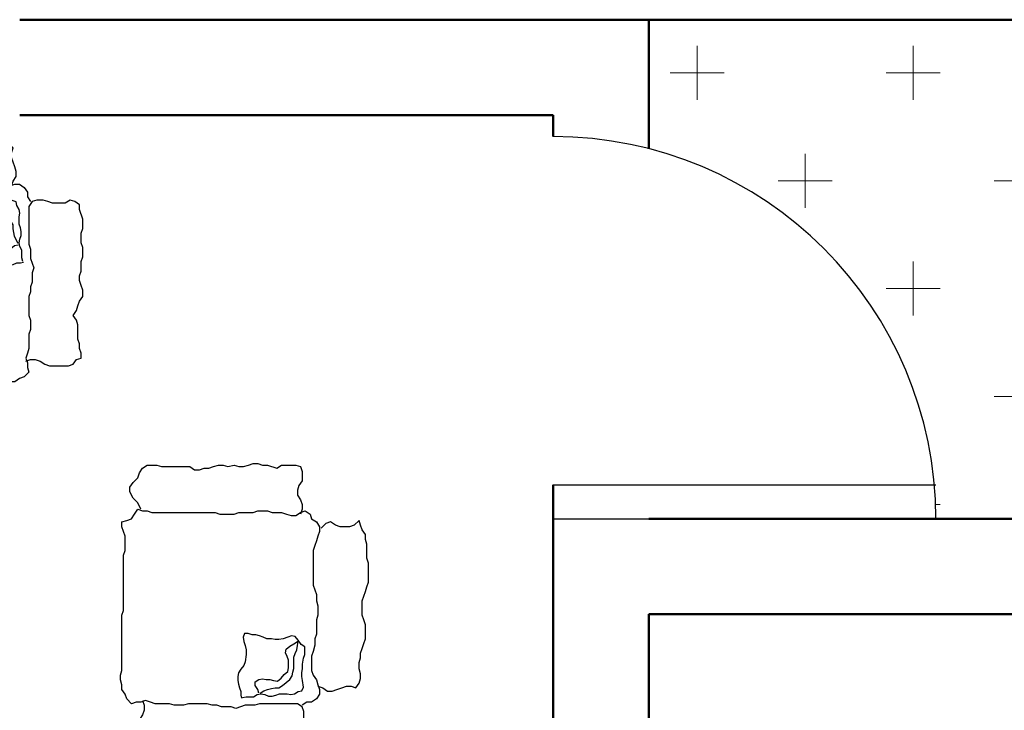
# Model space of a CAD drawing. Units: millimetres. Extents: x -857 to 54106, y -13666 to 13947.
# Tile 28 of 41: x 28540 to 30856, y 11178 to 12804. Entities that reach past the tile are written whole.
import ezdxf

# ---------------------------------------------------------------- set-up
doc = ezdxf.new("R2010")
doc.units = ezdxf.units.MM
for name, color, linetype, lineweight in [('A-DOOR', 1, 'Continuous', 25), ('A-FLOR-PATT', 252, 'Continuous', 13), ('A-FURN', 21, 'Continuous', 18), ('A-WALL', 7, 'Continuous', 50)]:
    doc.layers.add(name, color=color, linetype=linetype, lineweight=lineweight)
doc.layers.add('TEFRIŞ', color=11, linetype='Continuous')

# ---------------------------------------------------------------- blocks, each defined once
blk = doc.blocks.new('24')
at = {"layer": 'TEFRIŞ'}
for p, q in [((-1851.9, -153.78), (-1851.9, -152.78)), ((-1851.9, -152.78), (-1850.24, -152.78)), ((-1849.09, -151.25), (-1850.56, -152.23)), ((-1850.24, -152.78), (-1850.24, -152.11)), ((-1847.61, -151.25), (-1849.09, -151.25)), ((-1846.13, -150.75), (-1847.61, -151.25)), ((-1841.7, -150.75), (-1846.13, -150.75)), ((-1840.23, -150.26), (-1841.7, -150.75)), ((-1834.32, -150.26), (-1840.23, -150.26)), ((-1832.84, -150.75), (-1834.32, -150.26)), ((-1831.36, -151.25), (-1832.84, -150.75)), ((-1829.89, -151.74), (-1831.36, -151.25)), ((-1828.41, -152.23), (-1829.89, -151.74)), ((-1823.98, -152.23), (-1828.41, -152.23)), ((-1822.5, -151.74), (-1823.98, -152.23)), ((-1821.03, -151.25), (-1822.5, -151.74)), ((-1816.6, -151.25), (-1821.03, -151.25)), ((-1815.12, -151.74), (-1816.6, -151.25)), ((-1813.64, -152.23), (-1815.12, -151.74)), ((-1812.17, -152.72), (-1813.64, -152.23)), ((-1810.69, -152.72), (-1812.17, -152.72)), ((-1809.21, -153.21), (-1810.69, -152.72)), ((-1807.24, -153.21), (-1809.21, -153.21)), ((-1805.77, -152.72), (-1807.24, -153.21)), ((-1804.29, -152.72), (-1805.77, -152.72)), ((-1802.81, -153.21), (-1804.29, -152.72)), ((-1802.01, -153.28), (-1802.01, -152.88)), ((-1802.01, -152.88), (-1801, -152.88)), ((-1801, -152.88), (-1801, -152.68)), ((-1801, -152.68), (-1800, -152.68)), ((-1800, -152.68), (-1800, -152.48)), ((-1800, -152.48), (-1797.79, -152.48)), ((-1797.79, -152.48), (-1797.79, -152.68)), ((-1797.79, -152.68), (-1796.79, -152.68)), ((-1796.79, -152.68), (-1796.79, -153.08)), ((-1796.79, -153.08), (-1795.78, -153.08)), ((-1795.78, -153.08), (-1795.78, -152.68)), ((-1795.78, -152.68), (-1794.78, -152.68)), ((-1794.78, -152.68), (-1794.78, -152.08)), ((-1794.78, -152.08), (-1792.77, -152.08)), ((-1792.77, -152.08), (-1792.77, -152.68)), ((-1792.77, -152.68), (-1792.57, -152.68)), ((-1792.5, -152.78), (-1790.84, -152.78)), ((-1792.5, -153.78), (-1792.5, -152.78)), ((-1789.69, -151.25), (-1791.16, -152.23)), ((-1790.84, -152.78), (-1790.84, -152.11)), ((-1788.21, -151.25), (-1789.69, -151.25)), ((-1786.73, -150.75), (-1788.21, -151.25)), ((-1782.3, -150.75), (-1786.73, -150.75)), ((-1780.83, -150.26), (-1782.3, -150.75)), ((-1774.92, -150.26), (-1780.83, -150.26)), ((-1773.44, -150.75), (-1774.92, -150.26)), ((-1771.96, -151.25), (-1773.44, -150.75)), ((-1770.49, -151.74), (-1771.96, -151.25)), ((-1769.01, -152.23), (-1770.49, -151.74)), ((-1764.58, -152.23), (-1769.01, -152.23)), ((-1763.1, -151.74), (-1764.58, -152.23)), ((-1761.63, -151.25), (-1763.1, -151.74)), ((-1757.2, -151.25), (-1761.63, -151.25)), ((-1755.72, -151.74), (-1757.2, -151.25)), ((-1754.24, -152.23), (-1755.72, -151.74)), ((-1752.77, -152.72), (-1754.24, -152.23)), ((-1751.29, -152.72), (-1752.77, -152.72)), ((-1749.81, -153.21), (-1751.29, -152.72)), ((-1747.84, -153.21), (-1749.81, -153.21)), ((-1746.37, -152.72), (-1747.84, -153.21)), ((-1744.89, -152.72), (-1746.37, -152.72)), ((-1743.41, -153.21), (-1744.89, -152.72)), ((-1741.94, -154.2), (-1743.41, -153.21)), ((-1733.14, -152.78), (-1733.14, -153.45)), ((-1732.14, -152.78), (-1733.14, -152.78)), ((-1732.14, -152.45), (-1732.14, -152.78)), ((-1730.14, -152.45), (-1732.14, -152.45)), ((-1728.32, -151.25), (-1729.8, -152.23)), ((-1726.85, -151.25), (-1728.32, -151.25)), ((-1725.37, -150.75), (-1726.85, -151.25)), ((-1720.94, -150.75), (-1725.37, -150.75)), ((-1719.46, -150.26), (-1720.94, -150.75)), ((-1713.56, -150.26), (-1719.46, -150.26)), ((-1712.08, -150.75), (-1713.56, -150.26)), ((-1710.6, -151.25), (-1712.08, -150.75)), ((-1709.12, -151.74), (-1710.6, -151.25)), ((-1707.65, -152.23), (-1709.12, -151.74)), ((-1703.22, -152.23), (-1707.65, -152.23)), ((-1701.74, -151.74), (-1703.22, -152.23)), ((-1700.26, -151.25), (-1701.74, -151.74)), ((-1695.83, -151.25), (-1700.26, -151.25)), ((-1694.36, -151.74), (-1695.83, -151.25)), ((-1692.88, -152.23), (-1694.36, -151.74)), ((-1691.4, -152.72), (-1692.88, -152.23)), ((-1689.93, -152.72), (-1691.4, -152.72)), ((-1688.45, -153.21), (-1689.93, -152.72)), ((-1686.48, -153.21), (-1688.45, -153.21)), ((-1685, -152.72), (-1686.48, -153.21)), ((-1683.53, -152.72), (-1685, -152.72)), ((-1682.05, -153.21), (-1683.53, -152.72)), ((-1680.57, -154.2), (-1682.05, -153.21)), ((-1852.57, -156.78), (-1852.57, -155.78)), ((-1852.57, -155.78), (-1852.24, -155.78)), ((-1852.24, -155.78), (-1852.24, -153.78)), ((-1852.24, -153.78), (-1851.9, -153.78)), ((-1803.01, -153.28), (-1802.01, -153.28)), ((-1793.17, -155.78), (-1792.84, -155.78)), ((-1793.17, -156.78), (-1793.17, -155.78)), ((-1792.84, -155.78), (-1792.84, -153.78)), ((-1792.84, -153.78), (-1792.5, -153.78)), ((-1741.14, -154.45), (-1741.14, -154.11)), ((-1740.14, -154.45), (-1741.14, -154.45)), ((-1740.14, -155.11), (-1740.14, -154.45)), ((-1739.14, -155.11), (-1740.14, -155.11)), ((-1739.14, -155.45), (-1739.14, -155.11)), ((-1738.14, -155.45), (-1739.14, -155.45)), ((-1738.14, -155.11), (-1738.14, -155.45)), ((-1737.14, -155.11), (-1738.14, -155.11)), ((-1737.14, -154.45), (-1737.14, -155.11)), ((-1736.14, -154.45), (-1737.14, -154.45)), ((-1737.14, -155.45), (-1737.14, -155.11)), ((-1736.81, -155.45), (-1737.14, -155.45)), ((-1736.81, -157.45), (-1736.81, -155.45)), ((-1735.14, -154.11), (-1736.14, -154.11)), ((-1736.14, -154.11), (-1736.14, -154.45)), ((-1735.14, -153.78), (-1735.14, -154.11)), ((-1734.14, -153.78), (-1735.14, -153.78)), ((-1734.14, -153.45), (-1734.14, -153.78)), ((-1733.14, -153.45), (-1734.14, -153.45)), ((-1681.06, -155.67), (-1680.57, -154.2)), ((-1681.06, -157.15), (-1681.06, -155.67)), ((-1852.24, -156.78), (-1852.57, -156.78)), ((-1852.24, -158.78), (-1852.24, -156.78)), ((-1851.9, -158.78), (-1852.24, -158.78)), ((-1851.9, -162.78), (-1851.9, -158.78)), ((-1792.84, -156.78), (-1793.17, -156.78)), ((-1792.84, -158.78), (-1792.84, -156.78)), ((-1792.5, -158.78), (-1792.84, -158.78)), ((-1792.5, -162.78), (-1792.5, -158.78)), ((-1736.14, -157.45), (-1736.81, -157.45)), ((-1736.14, -158.45), (-1736.14, -157.45)), ((-1735.81, -158.45), (-1736.14, -158.45)), ((-1735.81, -160.11), (-1735.81, -158.45)), ((-1680.57, -158.63), (-1681.06, -157.15)), ((-1680.08, -160.1), (-1680.57, -158.63)), ((-1734.48, -160.11), (-1735.81, -160.11)), ((-1735.14, -162.11), (-1734.48, -162.11)), ((-1735.14, -163.11), (-1735.14, -162.11)), ((-1734.48, -162.11), (-1734.48, -160.11)), ((-1679.59, -161.58), (-1680.08, -160.1)), ((-1679.59, -163.05), (-1679.59, -161.58)), ((-1851.57, -162.78), (-1851.9, -162.78)), ((-1851.9, -166.44), (-1851.9, -165.44)), ((-1851.9, -165.44), (-1850.9, -165.44)), ((-1851.57, -164.78), (-1851.57, -162.78)), ((-1850.57, -164.78), (-1851.57, -164.78)), ((-1850.9, -165.44), (-1850.9, -164.78)), ((-1850.57, -165.44), (-1850.57, -164.78)), ((-1849.57, -165.44), (-1850.57, -165.44)), ((-1792.17, -162.78), (-1792.5, -162.78)), ((-1792.5, -165.44), (-1791.5, -165.44)), ((-1792.5, -166.44), (-1792.5, -165.44)), ((-1792.17, -164.78), (-1792.17, -162.78)), ((-1791.17, -164.78), (-1792.17, -164.78)), ((-1791.5, -165.44), (-1791.5, -164.78)), ((-1791.17, -165.44), (-1791.17, -164.78)), ((-1790.17, -165.44), (-1791.17, -165.44)), ((-1742.48, -164.78), (-1740.81, -164.78)), ((-1742.48, -165.78), (-1742.48, -164.78)), ((-1740.81, -164.11), (-1738.81, -164.11)), ((-1740.81, -164.78), (-1740.81, -164.11)), ((-1738.81, -164.11), (-1738.81, -164.45)), ((-1738.81, -164.45), (-1737.81, -164.45)), ((-1737.81, -164.45), (-1737.81, -164.78)), ((-1737.81, -164.78), (-1736.81, -164.78)), ((-1736.81, -164.78), (-1736.81, -165.11)), ((-1736.81, -165.11), (-1735.81, -165.11)), ((-1735.81, -165.44), (-1736.14, -165.44)), ((-1735.81, -163.11), (-1735.14, -163.11)), ((-1735.81, -165.11), (-1735.81, -163.11)), ((-1735.81, -165.11), (-1735.81, -165.44)), ((-1734.14, -165.11), (-1733.14, -165.11)), ((-1734.14, -165.78), (-1734.14, -165.11)), ((-1733.14, -164.78), (-1731.14, -164.78)), ((-1733.14, -165.11), (-1733.14, -164.78)), ((-1731.14, -164.78), (-1731.14, -165.11)), ((-1731.14, -165.11), (-1730.14, -165.11)), ((-1730.14, -165.11), (-1730.14, -165.44)), ((-1730.14, -165.44), (-1727.81, -165.44)), ((-1681.06, -166), (-1680.57, -164.53)), ((-1680.57, -164.53), (-1679.59, -163.05)), ((-1853.9, -169.44), (-1853.9, -168.44)), ((-1853.9, -168.44), (-1852.57, -168.44)), ((-1852.57, -168.44), (-1852.57, -166.44)), ((-1852.57, -166.44), (-1851.9, -166.44)), ((-1848.59, -166), (-1847.12, -166.5)), ((-1847.12, -166.5), (-1845.64, -166.99)), ((-1845.64, -166.99), (-1844.16, -167.48)), ((-1844.16, -167.48), (-1833.33, -167.48)), ((-1833.33, -167.48), (-1831.86, -166.99)), ((-1831.86, -166.99), (-1830.38, -166.5)), ((-1830.38, -166.5), (-1828.41, -166.5)), ((-1828.41, -166.5), (-1826.93, -166)), ((-1826.93, -166), (-1823.98, -166)), ((-1823.98, -166), (-1822.5, -166.5)), ((-1822.5, -166.5), (-1818.07, -166.5)), ((-1818.07, -166.5), (-1816.6, -166.99)), ((-1816.6, -166.99), (-1814.63, -166.99)), ((-1814.63, -166.99), (-1812.66, -167.48)), ((-1812.66, -167.48), (-1811.18, -167.97)), ((-1811.18, -167.97), (-1806.75, -167.97)), ((-1806.75, -167.97), (-1805.27, -167.48)), ((-1805.27, -167.48), (-1803.8, -166.5)), ((-1803.8, -166.5), (-1802.32, -166)), ((-1802.41, -166.32), (-1802.41, -165.92)), ((-1802.01, -166.32), (-1802.41, -166.32)), ((-1802.01, -166.72), (-1802.01, -166.32)), ((-1801, -166.72), (-1802.01, -166.72)), ((-1801, -166.92), (-1801, -166.72)), ((-1798.99, -166.92), (-1801, -166.92)), ((-1798.99, -167.12), (-1798.99, -166.92)), ((-1797.99, -167.12), (-1798.99, -167.12)), ((-1797.99, -167.72), (-1797.99, -167.12)), ((-1796.99, -167.72), (-1797.99, -167.72)), ((-1795.98, -167.52), (-1796.99, -167.52)), ((-1796.99, -167.52), (-1796.99, -167.72)), ((-1794.98, -167.12), (-1795.98, -167.12)), ((-1795.98, -167.12), (-1795.98, -167.52)), ((-1793.98, -166.72), (-1794.98, -166.72)), ((-1794.98, -166.72), (-1794.98, -167.12)), ((-1793.18, -168.92), (-1793.18, -167.92)), ((-1793.18, -167.92), (-1792.77, -167.92)), ((-1793.17, -166.44), (-1792.5, -166.44)), ((-1792.77, -167.92), (-1792.77, -166.32)), ((-1789.19, -166), (-1787.72, -166.5)), ((-1787.72, -166.5), (-1786.24, -166.99)), ((-1786.24, -166.99), (-1784.76, -167.48)), ((-1784.76, -167.48), (-1773.93, -167.48)), ((-1773.93, -167.48), (-1772.46, -166.99)), ((-1772.46, -166.99), (-1770.98, -166.5)), ((-1770.98, -166.5), (-1769.01, -166.5)), ((-1769.01, -166.5), (-1767.53, -166)), ((-1767.53, -166), (-1764.58, -166)), ((-1764.58, -166), (-1763.1, -166.5)), ((-1763.1, -166.5), (-1758.67, -166.5)), ((-1758.67, -166.5), (-1757.2, -166.99)), ((-1757.2, -166.99), (-1755.23, -166.99)), ((-1755.23, -166.99), (-1753.26, -167.48)), ((-1753.26, -167.48), (-1751.78, -167.97)), ((-1751.78, -167.97), (-1747.35, -167.97)), ((-1747.35, -167.97), (-1745.87, -167.48)), ((-1745.87, -167.48), (-1744.4, -166.5)), ((-1744.4, -166.5), (-1742.92, -166)), ((-1736.14, -165.78), (-1734.14, -165.78)), ((-1736.14, -166.11), (-1735.81, -166.11)), ((-1736.14, -169.44), (-1736.14, -166.11)), ((-1727.83, -166), (-1726.35, -166.5)), ((-1726.35, -166.5), (-1724.88, -166.99)), ((-1724.88, -166.99), (-1723.4, -167.48)), ((-1723.4, -167.48), (-1712.57, -167.48)), ((-1712.57, -167.48), (-1711.09, -166.99)), ((-1711.09, -166.99), (-1709.62, -166.5)), ((-1709.62, -166.5), (-1707.65, -166.5)), ((-1707.65, -166.5), (-1706.17, -166)), ((-1706.17, -166), (-1703.22, -166)), ((-1703.22, -166), (-1701.74, -166.5)), ((-1701.74, -166.5), (-1697.31, -166.5)), ((-1697.31, -166.5), (-1695.83, -166.99)), ((-1695.83, -166.99), (-1693.86, -166.99)), ((-1693.86, -166.99), (-1691.89, -167.48)), ((-1691.89, -167.48), (-1690.42, -167.97)), ((-1690.42, -167.97), (-1685.99, -167.97)), ((-1685.99, -167.97), (-1684.51, -167.48)), ((-1684.51, -167.48), (-1683.03, -166.5)), ((-1683.03, -166.5), (-1681.56, -166)), ((-1681.56, -166), (-1680.08, -165.51)), ((-1680.08, -165.51), (-1678.6, -165.51)), ((-1678.6, -165.51), (-1677.13, -166.5)), ((-1677.13, -166.5), (-1676.14, -167.97)), ((-1676.14, -167.97), (-1676.14, -169.45)), ((-1869.99, -172.89), (-1869.5, -171.42)), ((-1869.5, -171.42), (-1868.02, -170.92)), ((-1868.02, -170.92), (-1865.07, -170.92)), ((-1865.07, -170.92), (-1863.59, -171.91)), ((-1860.63, -172.4), (-1859.16, -171.42)), ((-1859.16, -171.42), (-1857.68, -170.92)), ((-1857.68, -170.92), (-1856.2, -170.92)), ((-1856.2, -170.92), (-1854.73, -171.42)), ((-1855.22, -171.42), (-1855.71, -169.94)), ((-1854.24, -172.89), (-1855.22, -171.42)), ((-1854.9, -169.44), (-1853.9, -169.44)), ((-1854.9, -170.78), (-1854.9, -169.44)), ((-1849.92, -172.16), (-1849.69, -171)), ((-1849.69, -171), (-1848.53, -170.54)), ((-1848.53, -170.54), (-1846.44, -170.77)), ((-1846.44, -170.77), (-1845.28, -171)), ((-1845.28, -171), (-1844.12, -171)), ((-1844.12, -171), (-1842.73, -170.77)), ((-1842.73, -170.77), (-1841.34, -170.77)), ((-1841.34, -170.77), (-1839.48, -170.54)), ((-1839.48, -170.54), (-1838.32, -170.07)), ((-1838.32, -170.07), (-1836, -170.07)), ((-1836, -170.07), (-1835.31, -171.23)), ((-1835.31, -171.23), (-1833.92, -172.16)), ((-1794.18, -171.93), (-1794.18, -170.93)), ((-1794.18, -170.93), (-1793.98, -170.93)), ((-1793.98, -170.93), (-1793.98, -169.93)), ((-1793.98, -169.93), (-1793.78, -169.93)), ((-1793.78, -169.93), (-1793.78, -168.92)), ((-1793.78, -168.92), (-1793.18, -168.92)), ((-1736.48, -174.11), (-1736.48, -169.44)), ((-1736.48, -169.44), (-1736.14, -169.44)), ((-1694.04, -171.23), (-1695.43, -172.16)), ((-1693.35, -170.07), (-1694.04, -171.23)), ((-1691.03, -170.07), (-1693.35, -170.07)), ((-1689.87, -170.54), (-1691.03, -170.07)), ((-1688.01, -170.77), (-1689.87, -170.54)), ((-1686.62, -170.77), (-1688.01, -170.77)), ((-1685.23, -171), (-1686.62, -170.77)), ((-1684.07, -171), (-1685.23, -171)), ((-1682.91, -170.77), (-1684.07, -171)), ((-1680.82, -170.54), (-1682.91, -170.77)), ((-1679.66, -171), (-1680.82, -170.54)), ((-1679.43, -172.16), (-1679.66, -171)), ((-1676.14, -169.45), (-1675.16, -170.92)), ((-1674.66, -170.92), (-1675.65, -172.4)), ((-1673.19, -170.43), (-1674.66, -170.92)), ((-1671.22, -170.43), (-1673.19, -170.43)), ((-1669.74, -170.92), (-1671.22, -170.43)), ((-1668.27, -171.42), (-1669.74, -170.92)), ((-1664.33, -171.42), (-1668.27, -171.42)), ((-1662.85, -170.43), (-1664.33, -171.42)), ((-1661.37, -170.92), (-1662.85, -170.43)), ((-1659.9, -171.91), (-1661.37, -170.92)), ((-1869.99, -177.32), (-1869.99, -172.89)), ((-1863.59, -171.91), (-1862.11, -172.4)), ((-1862.11, -172.4), (-1860.63, -172.4)), ((-1854.73, -175.84), (-1854.24, -174.37)), ((-1854.24, -174.37), (-1854.24, -172.89)), ((-1850.85, -174.48), (-1850.62, -173.32)), ((-1850.62, -175.64), (-1850.85, -174.48)), ((-1850.62, -173.32), (-1849.92, -172.16)), ((-1846.21, -174.71), (-1845.05, -174.01)), ((-1845.05, -174.01), (-1843.89, -173.78)), ((-1843.89, -173.78), (-1842.73, -173.55)), ((-1842.73, -173.55), (-1839.25, -173.55)), ((-1839.25, -173.55), (-1838.09, -173.09)), ((-1838.09, -173.09), (-1836.93, -172.62)), ((-1836.93, -172.62), (-1835.54, -172.39)), ((-1835.77, -174.71), (-1835.08, -173.55)), ((-1835.54, -172.39), (-1834.38, -172.16)), ((-1835.08, -173.55), (-1834.38, -172.39)), ((-1834.38, -172.39), (-1834.15, -171.93)), ((-1833.92, -172.16), (-1832.76, -173.09)), ((-1832.52, -174.25), (-1832.99, -175.4)), ((-1832.76, -173.09), (-1832.52, -174.25)), ((-1795.54, -174.11), (-1795.88, -174.11)), ((-1795.78, -173.94), (-1794.78, -173.94)), ((-1795.54, -176.44), (-1795.54, -174.11)), ((-1794.78, -173.94), (-1794.78, -171.93)), ((-1794.78, -171.93), (-1794.18, -171.93)), ((-1736.14, -174.11), (-1736.48, -174.11)), ((-1736.14, -176.44), (-1736.14, -174.11)), ((-1696.59, -173.09), (-1696.83, -174.25)), ((-1696.83, -174.25), (-1696.36, -175.4)), ((-1695.43, -172.16), (-1696.59, -173.09)), ((-1694.97, -172.39), (-1695.2, -171.93)), ((-1693.81, -172.39), (-1694.97, -172.16)), ((-1694.27, -173.55), (-1694.97, -172.39)), ((-1693.58, -174.71), (-1694.27, -173.55)), ((-1692.42, -172.62), (-1693.81, -172.39)), ((-1691.26, -173.09), (-1692.42, -172.62)), ((-1690.1, -173.55), (-1691.26, -173.09)), ((-1686.62, -173.55), (-1690.1, -173.55)), ((-1685.46, -173.78), (-1686.62, -173.55)), ((-1684.3, -174.01), (-1685.46, -173.78)), ((-1683.14, -174.71), (-1684.3, -174.01)), ((-1678.73, -173.32), (-1679.43, -172.16)), ((-1678.5, -174.48), (-1678.73, -173.32)), ((-1678.73, -175.64), (-1678.5, -174.48)), ((-1675.65, -172.4), (-1675.65, -184.21)), ((-1659.9, -173.38), (-1659.9, -171.91)), ((-1658.91, -176.34), (-1659.9, -173.38)), ((-1869, -178.8), (-1869.99, -177.32)), ((-1855.22, -177.32), (-1854.73, -175.84)), ((-1855.22, -180.27), (-1855.22, -177.32)), ((-1850.62, -177.95), (-1850.62, -175.64)), ((-1848.76, -178.19), (-1848.07, -177.03)), ((-1848.07, -177.03), (-1847.14, -175.87)), ((-1847.14, -175.87), (-1846.21, -174.71)), ((-1846.67, -178.65), (-1845.75, -177.49)), ((-1845.75, -177.49), (-1844.59, -176.56)), ((-1844.59, -176.56), (-1843.66, -175.4)), ((-1843.66, -175.4), (-1842.5, -175.17)), ((-1842.5, -175.17), (-1840.18, -175.17)), ((-1840.18, -175.17), (-1839.02, -175.64)), ((-1839.02, -175.64), (-1837.86, -176.1)), ((-1837.86, -176.1), (-1836.7, -175.87)), ((-1836.7, -175.87), (-1835.77, -174.71)), ((-1833.45, -176.8), (-1833.68, -178.19)), ((-1832.99, -175.4), (-1833.45, -176.8)), ((-1795.88, -178.44), (-1795.88, -176.44)), ((-1795.88, -176.44), (-1795.54, -176.44)), ((-1736.48, -178.44), (-1736.48, -176.44)), ((-1736.48, -176.44), (-1736.14, -176.44)), ((-1696.36, -175.4), (-1695.9, -176.8)), ((-1695.9, -176.8), (-1695.67, -178.19)), ((-1692.65, -175.87), (-1693.58, -174.71)), ((-1691.49, -176.1), (-1692.65, -175.87)), ((-1690.33, -175.64), (-1691.49, -176.1)), ((-1689.17, -175.17), (-1690.33, -175.64)), ((-1686.85, -175.17), (-1689.17, -175.17)), ((-1685.69, -175.4), (-1686.85, -175.17)), ((-1684.76, -176.56), (-1685.69, -175.4)), ((-1683.6, -177.49), (-1684.76, -176.56)), ((-1682.68, -178.65), (-1683.6, -177.49)), ((-1682.21, -175.87), (-1683.14, -174.71)), ((-1681.28, -177.03), (-1682.21, -175.87)), ((-1680.59, -178.19), (-1681.28, -177.03)), ((-1678.73, -177.95), (-1678.73, -175.64)), ((-1658.91, -179.29), (-1658.91, -176.34)), ((-1869.99, -181.75), (-1869, -178.8)), ((-1855.71, -181.75), (-1855.22, -180.27)), ((-1851.31, -180.27), (-1851.08, -179.11)), ((-1851.31, -181.43), (-1851.31, -180.27)), ((-1851.08, -179.11), (-1850.62, -177.95)), ((-1849.23, -181.66), (-1848.99, -180.5)), ((-1848.99, -180.5), (-1848.76, -179.35)), ((-1848.76, -179.35), (-1848.76, -178.19)), ((-1846.44, -179.81), (-1846.67, -178.65)), ((-1846.21, -180.97), (-1846.44, -179.81)), ((-1833.68, -178.19), (-1833.68, -179.35)), ((-1833.68, -179.35), (-1833.45, -180.5)), ((-1833.45, -180.5), (-1833.45, -181.9)), ((-1796.54, -186.77), (-1796.54, -180.44)), ((-1796.54, -180.44), (-1796.21, -180.44)), ((-1796.21, -180.44), (-1796.21, -178.44)), ((-1796.21, -178.44), (-1795.88, -178.44)), ((-1737.14, -180.44), (-1736.81, -180.44)), ((-1737.14, -186.77), (-1737.14, -180.44)), ((-1736.81, -178.44), (-1736.48, -178.44)), ((-1736.81, -180.44), (-1736.81, -178.44)), ((-1695.67, -179.35), (-1695.9, -180.5)), ((-1695.9, -180.5), (-1695.9, -181.9)), ((-1695.67, -178.19), (-1695.67, -179.35)), ((-1683.14, -180.97), (-1682.91, -179.81)), ((-1682.91, -179.81), (-1682.68, -178.65)), ((-1680.59, -179.35), (-1680.59, -178.19)), ((-1680.36, -180.5), (-1680.59, -179.35)), ((-1680.12, -181.66), (-1680.36, -180.5)), ((-1678.27, -179.11), (-1678.73, -177.95)), ((-1678.04, -180.27), (-1678.27, -179.11)), ((-1678.04, -181.43), (-1678.04, -180.27)), ((-1659.4, -180.76), (-1658.91, -179.29)), ((-1659.4, -183.71), (-1659.4, -180.76)), ((-1870.48, -184.7), (-1869.99, -183.22)), ((-1869.99, -183.22), (-1869.99, -181.75)), ((-1855.71, -184.7), (-1855.71, -181.75)), ((-1850.85, -182.59), (-1851.31, -181.43)), ((-1850.62, -183.75), (-1850.85, -182.59)), ((-1850.85, -184.91), (-1850.62, -183.75)), ((-1850.39, -183.98), (-1849.69, -182.82)), ((-1849.69, -182.82), (-1849.23, -181.66)), ((-1846.21, -182.13), (-1846.21, -180.97)), ((-1845.98, -183.29), (-1846.21, -182.13)), ((-1846.21, -184.45), (-1845.98, -183.29)), ((-1833.45, -181.9), (-1832.99, -183.05)), ((-1832.99, -183.05), (-1832.52, -184.21)), ((-1696.36, -183.05), (-1696.83, -184.21)), ((-1695.9, -181.9), (-1696.36, -183.05)), ((-1683.37, -183.29), (-1683.14, -182.13)), ((-1683.14, -184.45), (-1683.37, -183.29)), ((-1683.14, -182.13), (-1683.14, -180.97)), ((-1679.66, -182.82), (-1680.12, -181.66)), ((-1678.97, -183.98), (-1679.66, -182.82)), ((-1678.73, -183.75), (-1678.5, -182.59)), ((-1678.5, -184.91), (-1678.73, -183.75)), ((-1678.5, -182.59), (-1678.04, -181.43)), ((-1658.91, -185.19), (-1659.4, -183.71)), ((-1870.48, -186.17), (-1870.48, -184.7)), ((-1869.99, -187.65), (-1870.48, -186.17)), ((-1855.22, -186.17), (-1855.71, -184.7)), ((-1855.22, -190.6), (-1855.22, -186.17)), ((-1851.55, -186.07), (-1850.85, -184.91)), ((-1851.55, -188.39), (-1851.55, -186.07)), ((-1850.39, -184.45), (-1849.23, -184.68)), ((-1849.23, -184.68), (-1848.07, -185.6)), ((-1848.07, -185.6), (-1846.91, -185.6)), ((-1846.91, -185.6), (-1846.21, -184.45)), ((-1832.52, -184.21), (-1832.29, -185.37)), ((-1832.29, -185.37), (-1832.29, -186.53)), ((-1832.29, -186.53), (-1831.83, -187.69)), ((-1796.88, -189.77), (-1796.88, -186.77)), ((-1796.88, -186.77), (-1796.54, -186.77)), ((-1737.48, -186.77), (-1737.14, -186.77)), ((-1737.48, -189.77), (-1737.48, -186.77)), ((-1697.06, -186.53), (-1697.52, -187.69)), ((-1696.83, -184.21), (-1697.06, -185.37)), ((-1697.06, -185.37), (-1697.06, -186.53)), ((-1682.44, -185.6), (-1683.14, -184.45)), ((-1681.28, -185.6), (-1682.44, -185.6)), ((-1680.12, -184.68), (-1681.28, -185.6)), ((-1678.97, -184.45), (-1680.12, -184.68)), ((-1677.81, -186.07), (-1678.5, -184.91)), ((-1677.81, -188.39), (-1677.81, -186.07)), ((-1675.65, -184.21), (-1675.16, -185.68)), ((-1675.16, -185.68), (-1675.16, -188.63)), ((-1658.91, -188.14), (-1658.91, -185.19)), ((-1869.5, -189.13), (-1869.99, -187.65)), ((-1869.5, -190.6), (-1869.5, -189.13)), ((-1851.08, -190.01), (-1852.01, -189.78)), ((-1851.78, -189.54), (-1851.55, -188.39)), ((-1841.8, -189.08), (-1842.96, -190.01)), ((-1840.64, -188.62), (-1841.8, -189.08)), ((-1838.32, -188.39), (-1840.64, -188.62)), ((-1836.93, -188.39), (-1838.32, -188.39)), ((-1835.54, -188.62), (-1836.93, -188.39)), ((-1834.38, -189.08), (-1835.54, -188.62)), ((-1832.99, -189.31), (-1834.38, -189.08)), ((-1831.83, -188.85), (-1832.99, -189.31)), ((-1831.83, -187.69), (-1831.83, -188.85)), ((-1797.21, -199.44), (-1797.21, -189.77)), ((-1797.21, -189.77), (-1796.88, -189.77)), ((-1737.81, -189.77), (-1737.48, -189.77)), ((-1737.81, -199.44), (-1737.81, -189.77)), ((-1697.52, -187.69), (-1697.52, -188.85)), ((-1697.52, -188.85), (-1696.36, -189.31)), ((-1696.36, -189.31), (-1694.97, -189.08)), ((-1694.97, -189.08), (-1693.81, -188.62)), ((-1693.81, -188.62), (-1692.42, -188.39)), ((-1692.42, -188.39), (-1691.03, -188.39)), ((-1691.03, -188.39), (-1688.71, -188.62)), ((-1688.71, -188.62), (-1687.55, -189.08)), ((-1687.55, -189.08), (-1686.39, -190.01)), ((-1678.27, -190.01), (-1677.34, -189.78)), ((-1677.57, -189.54), (-1677.81, -188.39)), ((-1675.16, -188.63), (-1674.66, -190.11)), ((-1659.4, -189.62), (-1658.91, -188.14)), ((-1659.4, -192.57), (-1659.4, -189.62)), ((-1869.99, -192.08), (-1869.5, -190.6)), ((-1869.5, -194.05), (-1869.99, -192.08)), ((-1854.73, -192.08), (-1855.22, -190.6)), ((-1854.73, -196.51), (-1854.73, -192.08)), ((-1849.92, -190.01), (-1851.08, -190.01)), ((-1848.76, -190.47), (-1849.92, -190.01)), ((-1847.6, -190.7), (-1848.76, -190.47)), ((-1846.44, -190.94), (-1847.6, -190.7)), ((-1845.28, -190.94), (-1846.44, -190.94)), ((-1844.12, -190.7), (-1845.28, -190.94)), ((-1842.96, -190.01), (-1844.12, -190.7)), ((-1686.39, -190.01), (-1685.23, -190.7)), ((-1685.23, -190.7), (-1684.07, -190.94)), ((-1684.07, -190.94), (-1682.91, -190.94)), ((-1682.91, -190.94), (-1681.75, -190.7)), ((-1681.75, -190.7), (-1680.59, -190.47)), ((-1680.59, -190.47), (-1679.43, -190.01)), ((-1679.43, -190.01), (-1678.27, -190.01)), ((-1674.66, -190.11), (-1674.17, -191.59)), ((-1674.17, -191.59), (-1674.66, -193.06)), ((-1659.9, -194.05), (-1659.4, -192.57)), ((-1869.99, -195.52), (-1869.5, -194.05)), ((-1869.99, -197), (-1869.99, -195.52)), ((-1674.66, -196.01), (-1675.16, -197.49)), ((-1674.66, -193.06), (-1674.66, -196.01)), ((-1659.9, -195.52), (-1659.9, -194.05)), ((-1659.4, -197), (-1659.9, -195.52)), ((-1869.5, -198.47), (-1869.99, -197)), ((-1869, -199.95), (-1869.5, -198.47)), ((-1855.22, -197.98), (-1854.73, -196.51)), ((-1855.22, -217.66), (-1855.22, -197.98)), ((-1675.16, -198.97), (-1675.65, -200.44)), ((-1675.16, -197.49), (-1675.16, -198.97)), ((-1658.91, -198.47), (-1659.4, -197)), ((-1658.91, -200.44), (-1658.91, -198.47)), ((-1869, -201.43), (-1869, -199.95)), ((-1868.51, -202.9), (-1869, -201.43)), ((-1796.88, -199.44), (-1797.21, -199.44)), ((-1796.88, -201.44), (-1796.88, -199.44)), ((-1796.54, -201.44), (-1796.88, -201.44)), ((-1796.54, -205.44), (-1796.54, -201.44)), ((-1737.48, -199.44), (-1737.81, -199.44)), ((-1737.48, -201.44), (-1737.48, -199.44)), ((-1737.14, -201.44), (-1737.48, -201.44)), ((-1737.14, -205.44), (-1737.14, -201.44)), ((-1675.65, -200.44), (-1675.65, -206.34)), ((-1660.39, -203.39), (-1659.9, -201.92)), ((-1659.9, -201.92), (-1658.91, -200.44)), ((-1869.5, -205.85), (-1868.51, -204.38)), ((-1868.51, -204.38), (-1868.51, -202.9)), ((-1661.87, -206.34), (-1660.88, -204.87)), ((-1660.88, -204.87), (-1660.39, -203.39)), ((-1869.5, -214.71), (-1869.5, -205.85)), ((-1796.21, -205.44), (-1796.54, -205.44)), ((-1796.21, -207.44), (-1796.21, -205.44)), ((-1795.88, -207.44), (-1796.21, -207.44)), ((-1795.88, -208.44), (-1795.88, -207.44)), ((-1736.81, -205.44), (-1737.14, -205.44)), ((-1736.81, -207.44), (-1736.81, -205.44)), ((-1736.48, -207.44), (-1736.81, -207.44)), ((-1736.48, -208.44), (-1736.48, -207.44)), ((-1675.65, -206.34), (-1675.16, -207.82)), ((-1675.16, -207.82), (-1675.16, -210.77)), ((-1660.88, -207.82), (-1661.87, -206.34)), ((-1660.39, -209.3), (-1660.88, -207.82)), ((-1795.21, -208.44), (-1795.88, -208.44)), ((-1795.21, -209.44), (-1795.21, -208.44)), ((-1794.88, -209.44), (-1795.21, -209.44)), ((-1794.88, -210.77), (-1794.88, -209.44)), ((-1794.54, -210.77), (-1794.88, -210.77)), ((-1794.54, -211.77), (-1794.54, -210.77)), ((-1735.81, -208.44), (-1736.48, -208.44)), ((-1735.81, -209.44), (-1735.81, -208.44)), ((-1735.48, -209.44), (-1735.81, -209.44)), ((-1735.48, -210.77), (-1735.48, -209.44)), ((-1735.14, -210.77), (-1735.48, -210.77)), ((-1735.14, -211.77), (-1735.14, -210.77)), ((-1675.16, -210.77), (-1675.65, -212.25)), ((-1660.39, -213.72), (-1660.39, -209.3)), ((-1794.21, -211.77), (-1794.54, -211.77)), ((-1794.21, -213.77), (-1794.21, -211.77)), ((-1793.87, -213.77), (-1794.21, -213.77)), ((-1793.87, -215.1), (-1793.87, -213.77)), ((-1734.81, -211.77), (-1735.14, -211.77)), ((-1734.81, -213.77), (-1734.81, -211.77)), ((-1734.48, -213.77), (-1734.81, -213.77)), ((-1734.48, -215.1), (-1734.48, -213.77)), ((-1675.65, -212.25), (-1675.65, -216.68)), ((-1659.9, -215.2), (-1660.39, -213.72)), ((-1869.99, -216.18), (-1869.5, -214.71)), ((-1869.99, -219.14), (-1869.99, -216.18)), ((-1793.54, -215.1), (-1793.87, -215.1)), ((-1793.87, -218.1), (-1793.87, -217.1)), ((-1793.87, -217.1), (-1793.54, -217.1)), ((-1793.54, -217.1), (-1793.54, -215.1)), ((-1734.14, -215.1), (-1734.48, -215.1)), ((-1734.48, -217.1), (-1734.14, -217.1)), ((-1734.48, -218.1), (-1734.48, -217.1)), ((-1734.14, -217.1), (-1734.14, -215.1)), ((-1675.65, -216.68), (-1676.14, -218.15)), ((-1659.9, -216.68), (-1659.9, -215.2)), ((-1659.4, -218.15), (-1659.9, -216.68)), ((-1869, -220.61), (-1869.99, -219.14)), ((-1867.53, -221.6), (-1869, -220.61)), ((-1856.2, -222.09), (-1855.71, -220.61)), ((-1855.71, -219.14), (-1855.22, -217.66)), ((-1855.71, -220.61), (-1855.71, -219.14)), ((-1794.21, -219.77), (-1794.21, -218.1)), ((-1794.21, -218.1), (-1793.87, -218.1)), ((-1736.48, -220.77), (-1736.48, -219.77)), ((-1736.48, -219.77), (-1734.81, -219.77)), ((-1734.81, -218.1), (-1734.48, -218.1)), ((-1734.81, -219.77), (-1734.81, -218.1)), ((-1676.14, -218.15), (-1676.63, -219.63)), ((-1676.63, -219.63), (-1676.14, -221.1)), ((-1676.63, -220.61), (-1675.16, -220.12)), ((-1675.16, -220.12), (-1673.68, -220.12)), ((-1673.68, -220.12), (-1672.2, -220.61)), ((-1672.2, -220.61), (-1670.73, -221.6)), ((-1661.87, -221.6), (-1660.88, -220.12)), ((-1660.88, -220.12), (-1659.4, -219.63)), ((-1659.4, -219.63), (-1659.4, -218.15)), ((-1866.05, -222.09), (-1867.53, -221.6)), ((-1864.57, -223.56), (-1866.05, -222.09)), ((-1863.1, -224.55), (-1864.57, -223.56)), ((-1859.65, -223.56), (-1861.62, -224.55)), ((-1858.17, -222.09), (-1859.65, -223.56)), ((-1856.2, -221.1), (-1858.17, -222.09)), ((-1854.49, -224.07), (-1855.96, -223.09)), ((-1796.21, -221.77), (-1796.21, -220.77)), ((-1796.21, -220.77), (-1795.88, -220.77)), ((-1795.9, -223.58), (-1795.41, -225.06)), ((-1736.81, -220.77), (-1736.48, -220.77)), ((-1736.81, -221.77), (-1736.81, -220.77)), ((-1736.5, -222.1), (-1736.5, -223.58)), ((-1736.5, -223.58), (-1736.01, -225.06)), ((-1734.72, -223.07), (-1736.2, -222.09)), ((-1733.25, -224.06), (-1734.72, -223.07)), ((-1676.14, -221.1), (-1676.14, -222.58)), ((-1676.14, -222.58), (-1675.65, -224.06)), ((-1670.73, -221.6), (-1669.25, -222.09)), ((-1669.25, -222.09), (-1663.34, -222.09)), ((-1663.34, -222.09), (-1661.87, -221.6)), ((-1853.01, -225.06), (-1854.49, -224.07)), ((-1852.52, -226.53), (-1853.01, -225.06)), ((-1852.02, -228.01), (-1852.52, -226.53)), ((-1796.89, -226.53), (-1798.37, -227.02)), ((-1795.41, -225.06), (-1796.89, -226.53)), ((-1793.61, -225.06), (-1795.09, -224.07)), ((-1793.12, -226.53), (-1793.61, -225.06)), ((-1792.62, -228.01), (-1793.12, -226.53)), ((-1737.49, -226.53), (-1738.97, -227.02)), ((-1736.01, -225.06), (-1737.49, -226.53)), ((-1732.75, -225.53), (-1733.25, -224.06)), ((-1732.26, -227.01), (-1732.75, -225.53)), ((-1729.31, -226.52), (-1730.79, -227.01)), ((-1727.83, -226.02), (-1729.31, -226.52)), ((-1723.4, -226.02), (-1727.83, -226.02)), ((-1721.92, -226.52), (-1723.4, -226.02)), ((-1704.69, -226.52), (-1721.92, -226.52)), ((-1703.22, -227.01), (-1704.69, -226.52)), ((-1678.6, -226.02), (-1680.08, -227.01)), ((-1677.13, -225.53), (-1678.6, -226.02)), ((-1675.65, -224.06), (-1677.13, -225.53)), ((-1850.55, -228.01), (-1852.02, -228.01)), ((-1849.07, -227.51), (-1850.55, -228.01)), ((-1847.59, -227.02), (-1849.07, -227.51)), ((-1843.16, -227.02), (-1847.59, -227.02)), ((-1841.69, -227.51), (-1843.16, -227.02)), ((-1824.46, -227.51), (-1841.69, -227.51)), ((-1822.98, -228.01), (-1824.46, -227.51)), ((-1805.75, -228.01), (-1822.98, -228.01)), ((-1804.27, -228.5), (-1805.75, -228.01)), ((-1802.8, -228.5), (-1804.27, -228.5)), ((-1801.32, -228.01), (-1802.8, -228.5)), ((-1799.84, -228.01), (-1801.32, -228.01)), ((-1798.37, -227.02), (-1799.84, -228.01)), ((-1791.15, -228.01), (-1792.62, -228.01)), ((-1789.67, -227.51), (-1791.15, -228.01)), ((-1788.19, -227.02), (-1789.67, -227.51)), ((-1783.76, -227.02), (-1788.19, -227.02)), ((-1782.29, -227.51), (-1783.76, -227.02)), ((-1765.06, -227.51), (-1782.29, -227.51)), ((-1763.58, -228.01), (-1765.06, -227.51)), ((-1746.35, -228.01), (-1763.58, -228.01)), ((-1744.87, -228.5), (-1746.35, -228.01)), ((-1743.4, -228.5), (-1744.87, -228.5)), ((-1741.92, -228.01), (-1743.4, -228.5)), ((-1740.44, -228.01), (-1741.92, -228.01)), ((-1738.97, -227.02), (-1740.44, -228.01)), ((-1730.79, -227.01), (-1732.26, -227.01)), ((-1685.99, -227.01), (-1703.22, -227.01)), ((-1684.51, -227.5), (-1685.99, -227.01)), ((-1683.03, -227.5), (-1684.51, -227.5)), ((-1681.56, -227.01), (-1683.03, -227.5)), ((-1680.08, -227.01), (-1681.56, -227.01))]:
    blk.add_line(p, q, dxfattribs=at)
blk = doc.blocks.new('25')
at = {"layer": 'TEFRIŞ'}
for p, q in [((-1948.17, -298.66), (-1948.67, -300.14)), ((-1948.67, -300.14), (-1948.67, -303.09)), ((-1946.7, -298.17), (-1948.17, -298.66)), ((-1942.27, -298.17), (-1946.7, -298.17)), ((-1940.79, -299.15), (-1942.27, -298.17)), ((-1937.84, -298.17), (-1940.79, -299.15)), ((-1936.37, -298.17), (-1937.84, -298.17)), ((-1934.89, -297.68), (-1936.37, -298.17)), ((-1933.42, -297.68), (-1934.89, -297.68)), ((-1931.94, -298.17), (-1933.42, -297.68)), ((-1930.46, -298.66), (-1931.94, -298.17)), ((-1928.99, -298.66), (-1930.46, -298.66)), ((-1927.51, -298.17), (-1928.99, -298.66)), ((-1925.54, -298.66), (-1927.51, -298.17)), ((-1924.07, -298.17), (-1925.54, -298.66)), ((-1922.59, -298.17), (-1924.07, -298.17)), ((-1921.12, -298.66), (-1922.59, -298.17)), ((-1919.64, -299.15), (-1921.12, -298.66)), ((-1918.16, -299.15), (-1919.64, -299.15)), ((-1916.69, -299.64), (-1918.16, -299.15)), ((-1915.21, -299.64), (-1916.69, -299.64)), ((-1913.74, -298.66), (-1915.21, -299.64)), ((-1904.88, -298.66), (-1913.74, -298.66)), ((-1903.41, -298.17), (-1904.88, -298.66)), ((-1900.45, -298.17), (-1903.41, -298.17)), ((-1898.98, -299.15), (-1900.45, -298.17)), ((-1897.99, -300.63), (-1898.98, -299.15)), ((-1948.67, -303.09), (-1947.68, -304.57)), ((-1897.5, -302.11), (-1897.99, -300.63)), ((-1896.03, -303.58), (-1897.5, -302.11)), ((-1947.68, -304.57), (-1947.19, -306.04)), ((-1947.19, -306.04), (-1947.19, -307.52)), ((-1895.04, -305.06), (-1896.03, -303.58)), ((-1895.04, -306.54), (-1895.04, -305.06)), ((-1948.17, -309), (-1948.67, -310.47)), ((-1947.19, -307.52), (-1948.17, -309)), ((-1897.5, -309.98), (-1896.03, -308.51)), ((-1896.03, -308.51), (-1895.04, -306.54)), ((-1949.65, -312.44), (-1951.13, -313.43)), ((-1948.17, -312.94), (-1949.65, -312.44)), ((-1948.67, -310.47), (-1948.67, -311.95)), ((-1948.67, -311.95), (-1948.17, -313.43)), ((-1937.84, -312.44), (-1939.32, -312.94)), ((-1934.89, -312.44), (-1937.84, -312.44)), ((-1933.42, -312.94), (-1934.89, -312.44)), ((-1900.45, -312.44), (-1901.93, -312.94)), ((-1898.98, -312.44), (-1900.45, -312.44)), ((-1897.5, -311.95), (-1898.98, -312.44)), ((-1898.49, -311.95), (-1897.5, -309.98)), ((-1896.52, -313.43), (-1897.5, -311.95)), ((-1966.87, -316.87), (-1966.38, -315.4)), ((-1966.38, -315.4), (-1964.9, -316.87)), ((-1951.62, -314.91), (-1953.09, -315.89)), ((-1951.13, -313.43), (-1951.62, -314.91)), ((-1946.7, -313.92), (-1948.17, -312.94)), ((-1945.22, -313.92), (-1946.7, -313.92)), ((-1943.75, -313.43), (-1945.22, -313.92)), ((-1942.27, -312.94), (-1943.75, -313.43)), ((-1939.32, -312.94), (-1942.27, -312.94)), ((-1928.99, -312.94), (-1933.42, -312.94)), ((-1927.51, -313.43), (-1928.99, -312.94)), ((-1923.08, -313.43), (-1927.51, -313.43)), ((-1921.61, -312.94), (-1923.08, -313.43)), ((-1901.93, -312.94), (-1921.61, -312.94)), ((-1895.53, -314.91), (-1896.52, -313.43)), ((-1894.06, -315.4), (-1895.53, -314.91)), ((-1892.58, -315.89), (-1894.06, -315.4)), ((-1968.34, -319.83), (-1967.36, -318.35)), ((-1967.36, -318.35), (-1966.87, -316.87)), ((-1964.9, -316.87), (-1963.42, -317.37)), ((-1963.42, -317.37), (-1960.47, -317.37)), ((-1960.47, -317.37), (-1959, -316.87)), ((-1959, -316.87), (-1957.52, -315.89)), ((-1957.52, -315.89), (-1956.05, -316.38)), ((-1956.05, -316.38), (-1954.57, -317.86)), ((-1953.09, -315.89), (-1954.08, -317.37)), ((-1954.08, -317.37), (-1954.08, -318.84)), ((-1893.08, -318.84), (-1892.58, -317.37)), ((-1892.58, -317.37), (-1892.58, -315.89)), ((-1968.84, -322.78), (-1968.34, -321.31)), ((-1968.34, -321.31), (-1968.34, -319.83)), ((-1954.08, -318.84), (-1953.59, -320.32)), ((-1953.59, -320.32), (-1953.09, -321.8)), ((-1893.57, -320.32), (-1893.08, -318.84)), ((-1893.57, -324.75), (-1893.57, -320.32)), ((-1968.84, -327.21), (-1968.84, -322.78)), ((-1953.09, -321.8), (-1952.6, -323.27)), ((-1952.6, -323.27), (-1952.11, -324.75)), ((-1952.11, -324.75), (-1952.11, -335.58)), ((-1893.08, -326.23), (-1893.57, -324.75)), ((-1969.33, -328.69), (-1968.84, -327.21)), ((-1893.08, -343.46), (-1893.08, -326.23)), ((-1969.33, -334.6), (-1969.33, -328.69)), ((-1968.84, -336.07), (-1969.33, -334.6)), ((-1968.34, -337.55), (-1968.84, -336.07)), ((-1952.6, -337.06), (-1953.09, -338.54)), ((-1952.11, -335.58), (-1952.6, -337.06)), ((-1967.85, -339.03), (-1968.34, -337.55)), ((-1967.36, -340.5), (-1967.85, -339.03)), ((-1953.09, -338.54), (-1953.09, -340.5)), ((-1967.36, -344.94), (-1967.36, -340.5)), ((-1953.09, -340.5), (-1953.59, -341.98)), ((-1953.59, -341.98), (-1953.59, -344.94)), ((-1967.85, -346.41), (-1967.36, -344.94)), ((-1953.59, -344.94), (-1953.09, -346.41)), ((-1892.58, -344.94), (-1893.08, -343.46)), ((-1892.58, -362.17), (-1892.58, -344.94)), ((-1968.34, -347.89), (-1967.85, -346.41)), ((-1968.34, -352.32), (-1968.34, -347.89)), ((-1953.09, -346.41), (-1953.09, -350.84)), ((-1967.85, -353.8), (-1968.34, -352.32)), ((-1953.09, -350.84), (-1952.6, -352.32)), ((-1952.6, -352.32), (-1952.6, -354.29)), ((-1947.43, -352.72), (-1946.5, -351.56)), ((-1946.5, -351.56), (-1945.34, -351.33)), ((-1945.34, -351.33), (-1944.19, -351.79)), ((-1944.19, -351.79), (-1942.79, -352.25)), ((-1942.79, -352.25), (-1941.4, -352.49)), ((-1940.24, -352.49), (-1939.09, -352.25)), ((-1939.09, -352.25), (-1937.69, -352.25)), ((-1937.69, -352.25), (-1936.54, -351.79)), ((-1936.54, -351.79), (-1935.38, -351.33)), ((-1935.38, -351.33), (-1934.22, -351.09)), ((-1934.22, -351.09), (-1933.06, -351.09)), ((-1933.06, -351.09), (-1931.9, -350.63)), ((-1931.9, -350.63), (-1930.74, -350.63)), ((-1930.74, -350.63), (-1930.28, -351.79)), ((-1930.28, -351.79), (-1930.51, -353.18)), ((-1967.36, -355.27), (-1967.85, -353.8)), ((-1966.87, -356.75), (-1967.36, -355.27)), ((-1952.6, -354.29), (-1952.11, -356.26)), ((-1949.52, -354.81), (-1948.36, -354.11)), ((-1949.52, -357.13), (-1949.52, -354.81)), ((-1948.36, -354.11), (-1947.43, -352.72)), ((-1947.2, -353.18), (-1947.66, -352.95)), ((-1947.2, -354.34), (-1947.43, -353.18)), ((-1946.04, -353.88), (-1947.2, -353.18)), ((-1946.97, -355.73), (-1947.2, -354.34)), ((-1944.88, -354.57), (-1946.04, -353.88)), ((-1943.72, -355.5), (-1944.88, -354.57)), ((-1941.4, -352.49), (-1940.24, -352.49)), ((-1930.97, -354.34), (-1931.2, -355.73)), ((-1930.51, -353.18), (-1930.97, -354.34)), ((-1966.87, -358.23), (-1966.87, -356.75)), ((-1966.38, -359.7), (-1966.87, -358.23)), ((-1952.11, -356.26), (-1951.62, -357.73)), ((-1951.62, -357.73), (-1951.62, -362.17)), ((-1949.05, -358.29), (-1949.52, -357.13)), ((-1948.82, -360.14), (-1949.05, -358.29)), ((-1946.5, -356.89), (-1946.97, -355.73)), ((-1946.04, -358.05), (-1946.5, -356.89)), ((-1946.04, -361.53), (-1946.04, -358.05)), ((-1944.42, -358.98), (-1943.95, -357.82)), ((-1943.95, -357.82), (-1943.49, -356.66)), ((-1943.49, -356.66), (-1943.72, -355.5)), ((-1931.2, -355.73), (-1931.2, -357.13)), ((-1931.2, -357.13), (-1930.97, -359.44)), ((-1966.38, -361.67), (-1966.38, -359.7)), ((-1948.82, -361.53), (-1948.82, -360.14)), ((-1948.59, -362.92), (-1948.82, -361.53)), ((-1945.81, -362.69), (-1946.04, -361.53)), ((-1944.42, -361.3), (-1944.42, -358.98)), ((-1944.19, -362.46), (-1944.42, -361.3)), ((-1930.97, -359.44), (-1930.51, -360.6)), ((-1930.51, -360.6), (-1929.58, -361.76)), ((-1966.87, -363.15), (-1966.38, -361.67)), ((-1966.87, -364.63), (-1966.87, -363.15)), ((-1966.38, -366.1), (-1966.87, -364.63)), ((-1952.11, -363.64), (-1953.09, -365.12)), ((-1951.62, -362.17), (-1952.11, -363.64)), ((-1948.82, -365.24), (-1948.59, -364.08)), ((-1948.59, -364.08), (-1948.59, -362.92)), ((-1945.58, -363.85), (-1945.81, -362.69)), ((-1944.88, -365.01), (-1945.58, -363.85)), ((-1943.03, -363.39), (-1944.19, -362.46)), ((-1942.1, -364.55), (-1943.03, -363.39)), ((-1940.94, -365.48), (-1942.1, -364.55)), ((-1929.58, -361.76), (-1928.89, -362.92)), ((-1928.89, -362.92), (-1928.65, -364.08)), ((-1928.65, -364.08), (-1928.65, -365.24)), ((-1892.09, -363.64), (-1892.58, -362.17)), ((-1892.09, -365.12), (-1892.09, -363.64)), ((-1965.39, -367.58), (-1966.38, -366.1)), ((-1963.92, -367.09), (-1965.39, -367.58)), ((-1962.44, -367.09), (-1963.92, -367.09)), ((-1960.97, -367.58), (-1962.44, -367.09)), ((-1959.49, -368.07), (-1960.97, -367.58)), ((-1955.06, -367.58), (-1956.54, -368.56)), ((-1953.59, -367.09), (-1955.06, -367.58)), ((-1953.59, -366.6), (-1954.08, -368.07)), ((-1953.09, -365.12), (-1953.59, -366.6)), ((-1949.05, -367.33), (-1948.82, -365.24)), ((-1948.59, -368.49), (-1949.05, -367.33)), ((-1943.72, -365.94), (-1944.88, -365.01)), ((-1942.56, -366.87), (-1943.72, -365.94)), ((-1941.4, -367.56), (-1942.56, -366.87)), ((-1940.24, -367.56), (-1941.4, -367.56)), ((-1939.78, -365.24), (-1940.94, -365.48)), ((-1939.09, -367.8), (-1940.24, -367.56)), ((-1938.62, -365.01), (-1939.78, -365.24)), ((-1937.46, -365.01), (-1938.62, -365.01)), ((-1936.3, -364.78), (-1937.46, -365.01)), ((-1935.14, -365.01), (-1936.3, -364.78)), ((-1933.99, -365.71), (-1935.14, -365.01)), ((-1934.91, -368.03), (-1933.99, -366.87)), ((-1933.99, -366.87), (-1933.99, -365.71)), ((-1929.12, -367.56), (-1929.58, -368.72)), ((-1928.89, -366.4), (-1929.12, -367.56)), ((-1928.65, -365.24), (-1928.89, -366.4)), ((-1892.58, -366.6), (-1892.09, -365.12)), ((-1892.58, -368.07), (-1892.58, -366.6)), ((-1958.01, -368.56), (-1959.49, -368.07)), ((-1956.54, -368.56), (-1958.01, -368.56)), ((-1954.08, -368.07), (-1954.08, -369.55)), ((-1954.08, -369.55), (-1953.09, -371.03)), ((-1947.43, -368.72), (-1948.59, -368.49)), ((-1946.27, -369.42), (-1947.43, -368.72)), ((-1945.11, -369.65), (-1946.27, -369.42)), ((-1943.95, -369.42), (-1945.11, -369.65)), ((-1941.64, -369.42), (-1943.95, -369.42)), ((-1940.48, -369.88), (-1941.64, -369.42)), ((-1939.32, -370.12), (-1940.48, -369.88)), ((-1938.16, -370.12), (-1939.32, -370.12)), ((-1937.93, -368.03), (-1939.09, -367.8)), ((-1937, -369.65), (-1938.16, -370.12)), ((-1936.77, -368.49), (-1937.93, -368.03)), ((-1935.84, -369.42), (-1937, -369.65)), ((-1935.61, -369.19), (-1936.77, -368.49)), ((-1934.68, -369.65), (-1935.84, -369.42)), ((-1935.14, -369.19), (-1934.91, -368.03)), ((-1933.52, -370.35), (-1934.68, -369.65)), ((-1931.2, -370.35), (-1933.52, -370.35)), ((-1930.05, -370.58), (-1931.2, -370.35)), ((-1929.58, -369.88), (-1929.81, -370.81)), ((-1929.58, -368.72), (-1929.58, -369.88)), ((-1894.06, -371.03), (-1893.57, -369.55)), ((-1893.57, -369.55), (-1892.58, -368.07)), ((-1953.09, -371.03), (-1951.62, -372.01)), ((-1951.62, -372.01), (-1950.14, -372.01)), ((-1950.14, -372.01), (-1948.67, -373)), ((-1949.16, -374.96), (-1948.67, -373.49)), ((-1948.67, -373.49), (-1947.19, -372.5)), ((-1947.19, -372.5), (-1935.38, -372.5)), ((-1935.38, -372.5), (-1933.91, -373)), ((-1933.91, -373), (-1930.96, -373)), ((-1930.96, -373), (-1929.48, -373.49)), ((-1929.48, -373.49), (-1928, -373.98)), ((-1928, -373.98), (-1926.53, -373.49)), ((-1926.53, -373.49), (-1923.58, -373.49)), ((-1923.58, -373.49), (-1922.1, -373)), ((-1922.1, -373), (-1920.62, -373)), ((-1920.62, -373), (-1919.15, -372.5)), ((-1919.15, -372.5), (-1913.25, -372.5)), ((-1913.25, -372.5), (-1911.77, -373)), ((-1911.77, -373), (-1908.82, -373)), ((-1908.82, -373), (-1907.34, -372.5)), ((-1907.34, -372.5), (-1902.91, -372.5)), ((-1902.91, -372.5), (-1901.44, -372.01)), ((-1901.44, -372.01), (-1899.96, -371.52)), ((-1899.96, -371.52), (-1898.49, -372.01)), ((-1898.98, -371.52), (-1899.47, -373)), ((-1899.47, -373), (-1899.47, -374.47)), ((-1898.49, -372.01), (-1897.01, -372.01)), ((-1897.01, -372.01), (-1895.53, -372.5)), ((-1895.53, -372.5), (-1894.06, -371.03)), ((-1949.16, -376.93), (-1949.16, -374.96)), ((-1899.47, -374.47), (-1898.98, -375.95)), ((-1898.98, -375.95), (-1897.99, -377.43)), ((-1948.67, -378.41), (-1949.16, -376.93)), ((-1948.17, -379.89), (-1948.67, -378.41)), ((-1948.17, -383.83), (-1948.17, -379.89)), ((-1897.99, -377.43), (-1897.5, -378.9)), ((-1897.5, -378.9), (-1897.5, -384.81)), ((-1949.16, -385.3), (-1948.17, -383.83)), ((-1948.67, -386.78), (-1949.16, -385.3)), ((-1897.5, -384.81), (-1897.99, -386.29)), ((-1947.68, -388.26), (-1948.67, -386.78)), ((-1946.21, -388.26), (-1947.68, -388.26)), ((-1943.25, -389.24), (-1946.21, -388.26)), ((-1938.83, -388.75), (-1940.3, -389.24)), ((-1935.88, -388.75), (-1938.83, -388.75)), ((-1934.4, -389.24), (-1935.88, -388.75)), ((-1929.97, -388.75), (-1931.45, -389.24)), ((-1927.02, -388.75), (-1929.97, -388.75)), ((-1925.54, -388.26), (-1927.02, -388.75)), ((-1924.07, -388.26), (-1925.54, -388.26)), ((-1922.59, -388.75), (-1924.07, -388.26)), ((-1921.12, -389.24), (-1922.59, -388.75)), ((-1917.67, -388.26), (-1919.15, -389.24)), ((-1916.2, -387.76), (-1917.67, -388.26)), ((-1914.72, -387.27), (-1916.2, -387.76)), ((-1913.25, -386.29), (-1914.72, -387.27)), ((-1911.77, -387.27), (-1913.25, -386.29)), ((-1910.29, -387.76), (-1911.77, -387.27)), ((-1905.87, -387.76), (-1910.29, -387.76)), ((-1904.39, -388.26), (-1905.87, -387.76)), ((-1902.91, -388.26), (-1904.39, -388.26)), ((-1901.44, -388.75), (-1902.91, -388.26)), ((-1899.96, -388.75), (-1901.44, -388.75)), ((-1899.47, -387.27), (-1899.96, -388.75)), ((-1897.99, -386.29), (-1899.47, -387.27)), ((-1940.3, -389.24), (-1943.25, -389.24)), ((-1931.45, -389.24), (-1934.4, -389.24)), ((-1919.15, -389.24), (-1921.12, -389.24))]:
    blk.add_line(p, q, dxfattribs=at)
blk = doc.blocks.new('DOOR-900')
blk.add_line((11417.3, 9811.5), (12317.3, 9811.5))
blk.add_arc((11417.3, 9811.5), 900, 0, 90)

msp = doc.modelspace()

# ---------------------------------------------------------------- hatches: boundary and pattern name
at = {"layer": 'A-FLOR-PATT'}
h = msp.add_hatch(dxfattribs=at)
h.set_pattern_fill('CROSS', color=256, scale=40)
h.set_pattern_definition([(0, (-5489.92, -2561.3), (254, 254), [127, -381]), (90, (-5426.42, -2624.8), (-254, 254), [127, -381])])
h.paths.add_polyline_path([(33845.086, 12804.231), (30020.079, 12804.231), (30020.079, 12500.311, -0.3418929), (30695.079, 11629.231), (33845.08, 11629.231)])

# ---------------------------------------------------------------- linework, layer by layer
at = {"layer": 'A-DOOR'}
msp.add_line((29795.079, 11708.89), (30695.079, 11708.89), dxfattribs=at)
at = {"layer": 'A-WALL'}
for p, q in [((28539.742, 12804.231), (30020.079, 12804.231)), ((30020.079, 12804.231), (30020.079, 12500.311)), ((30020.079, 12804.231), (33845.086, 12804.231)), ((28539.742, 12579.231), (29795.079, 12579.231)), ((29795.079, 12579.231), (29795.079, 12528.89)), ((29795.079, 11628.89), (29795.079, 11708.89)), ((29795.079, 11628.89), (29795.079, 9579.231)), ((29795.079, 11628.89), (29795.079, 11628.89)), ((30020.079, 11629.231), (31489.168, 11629.231)), ((30020.079, 11404.231), (31489.168, 11404.231)), ((30020.079, 11404.231), (30020.079, 9184.795))]:
    msp.add_line(p, q, dxfattribs=at)

# ---------------------------------------------------------------- block references
at = {"layer": 'A-DOOR'}
msp.add_blockref('DOOR-900', (18377.799, 1817.408), dxfattribs=at)
at = {"layer": 'A-FURN', "yscale": 7.559220362162901, "zscale": 7.559220362162901}
for name, p, xscale in [('24', (41228.064, 13667.813), 7.559220362162901), ('25', (14473.896, 14009.447), -7.559220362162901)]:
    msp.add_blockref(name, p, dxfattribs=dict(at, xscale=xscale))

doc.saveas('drawing.dxf')
